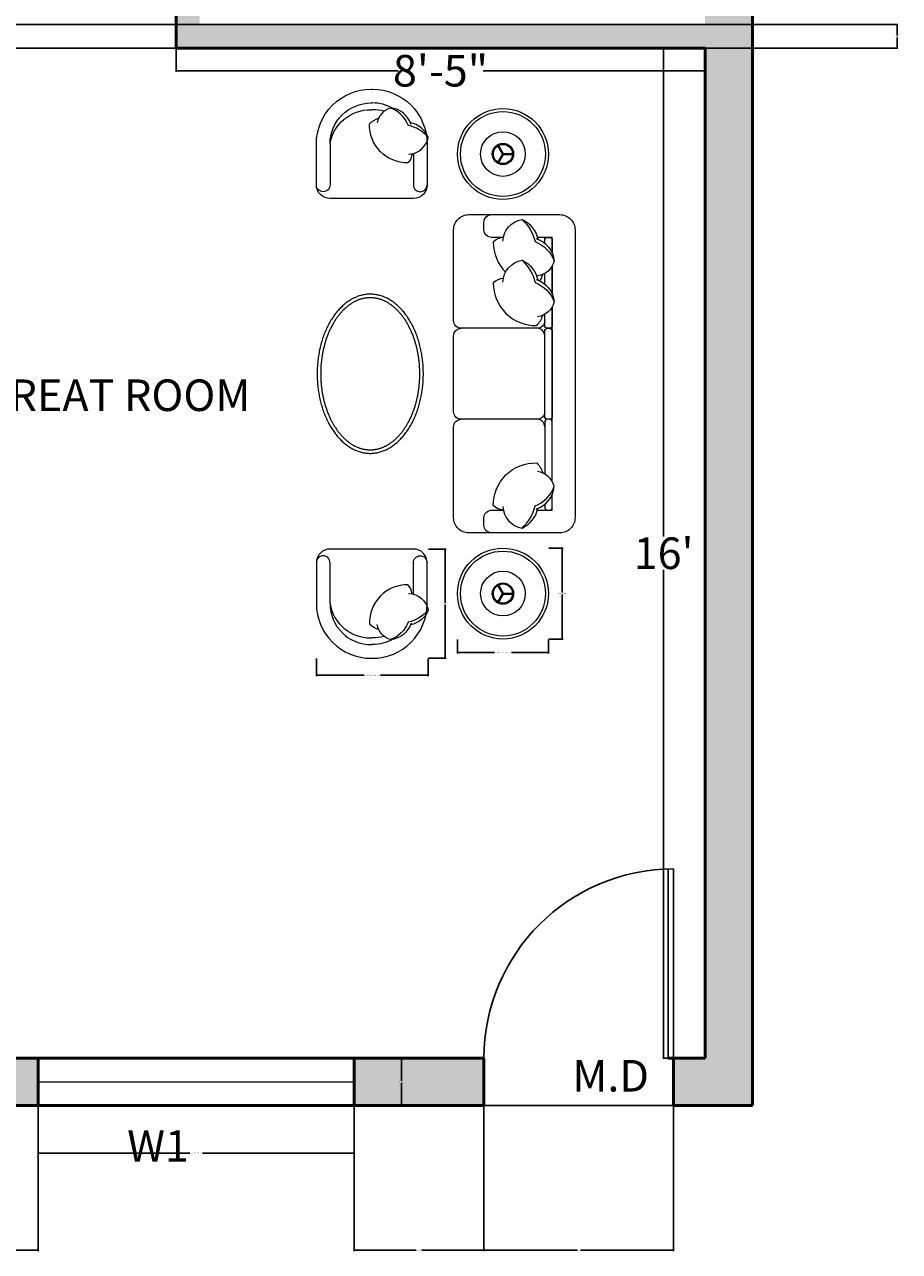
# Model space of a CAD drawing. Units: inches. Extents: x -22 to 470, y -437 to 97.
# Tile 4 of 9: x 304 to 470, y -425 to -192. Entities that reach past the tile are written whole.
import ezdxf

# ---------------------------------------------------------------- set-up
doc = ezdxf.new("R2010")
doc.units = ezdxf.units.IN
doc.header["$MEASUREMENT"] = 0
for name, color, linetype, lineweight in [('A-ANNO-DIMS', 2, 'Continuous', 18), ('A-ANNO-TEXT', 7, 'Continuous', 18), ('A-AREA-IDEN', 7, 'Continuous', 25), ('A-DOOR', 4, 'Continuous', 25), ('A-FURN', 8, 'Continuous', 18), ('A-GLAZ', 4, 'Continuous', 18), ('A-WALL', 7, 'Continuous', 50), ('A-WALL-PATT', 8, 'Continuous', 13)]:
    doc.layers.add(name, color=color, linetype=linetype, lineweight=lineweight)
doc.styles.get("Standard").update_dxf_attribs({"font": 'arial.ttf'})
doc.dimstyles.get("Standard").update_dxf_attribs({"dimtxt": 0.18, "dimasz": 0.18, "dimexe": 0.18, "dimexo": 0.0625, "dimgap": 0.09, "dimtad": 0, "dimtih": 1, "dimtoh": 1, "dimdec": 0, "dimzin": 0, "dimdsep": 46, "dimlunit": 3, "dimtxsty": 'Standard', "dimcen": 0.09, "dimadec": 0, "dimazin": 0, "dimtfac": 1, "dimtdec": 0, "dimtofl": 0, "dimtmove": 0, "dimatfit": 3, "dimfxl": 1, "dimtolj": 1, "dimtzin": 0, "dimarcsym": 0})

# ---------------------------------------------------------------- blocks, each defined once
blk = doc.blocks.new('*D21')
at = {"layer": 'A-ANNO-DIMS', "color": 0, "lineweight": -2, "transparency": 16777216}
for p, q in [((425.54, -196.94), (425.54, -289.6)), ((425.61, -196.76), (425.72, -196.76)), ((425.54, -388.58), (425.54, -295.91)), ((429.86, -388.76), (425.36, -388.76))]:
    blk.add_line(p, q, dxfattribs=at)
at = {"layer": 'A-ANNO-DIMS', "color": 0, "transparency": 16777216}
for points in [[(425.51, -196.94), (425.57, -196.94), (425.54, -196.76)], [(425.51, -388.58), (425.57, -388.58), (425.54, -388.76)]]:
    blk.add_solid(points, dxfattribs=at)
at = {"layer": 'Defpoints', "color": 0, "transparency": 16777216}
for p in [(425.54, -196.76), (425.54, -388.76), (429.92, -388.76)]:
    blk.add_point(p, dxfattribs=at)
at = {"layer": 'A-ANNO-DIMS', "color": 0, "transparency": 16777216, "insert": (425.54, -292.76), "char_height": 6, "attachment_point": 5}
blk.add_mtext("\\A1;16'", dxfattribs=at)
blk = doc.blocks.new('*D22')
at = {"layer": 'A-ANNO-DIMS', "color": 0, "lineweight": -2, "transparency": 16777216}
for p, q in [((332.92, -196.82), (332.92, -201.22)), ((433.42, -196.82), (433.42, -201.22)), ((333.1, -201.04), (375.1, -201.04)), ((433.24, -201.04), (391.24, -201.04))]:
    blk.add_line(p, q, dxfattribs=at)
at = {"layer": 'A-ANNO-DIMS', "color": 0, "transparency": 16777216}
for points in [[(333.1, -201.01), (333.1, -201.07), (332.92, -201.04)], [(433.24, -201.01), (433.24, -201.07), (433.42, -201.04)]]:
    blk.add_solid(points, dxfattribs=at)
at = {"layer": 'Defpoints', "color": 0, "transparency": 16777216}
for p in [(332.92, -196.76), (433.42, -196.76), (433.42, -201.04)]:
    blk.add_point(p, dxfattribs=at)
at = {"layer": 'A-ANNO-DIMS', "color": 0, "transparency": 16777216, "insert": (383.17, -201.04), "char_height": 6, "attachment_point": 5}
blk.add_mtext('\\A1;8\'-5"', dxfattribs=at)
blk = doc.blocks.new('ARMCHAIR')
at = {"ltscale": 0.03}
blk.add_lwpolyline([(10.52, 20.78), (2.6, 20.78, 0.414214), (0, 18.18), (0, 10.39, 0.414214), (10.39, 0), (10.52, 0), (10.65, 0, 0.414214), (21.04, 10.39), (21.04, 18.18, 0.414214), (18.44, 20.78), (10.52, 20.78)], format="xyb", dxfattribs=at)
for points in [[(2.6, 10.39), (2.6, 18.18, 0.414214), (1.3, 19.48), (1.3, 19.48, 0.414214), (0, 18.18)], [(18.44, 12.21), (18.44, 18.18, -0.414214), (19.74, 19.48), (19.74, 19.48, -0.414214), (21.04, 18.18)], [(18.19, 12.27, 0.165541), (17.38, 13.99, 0.425989), (10.09, 6.55, 0.121523), (11.82, 5.52, -7.115464)], [(17.53, 12.35, -0.356772), (21.25, 9.08, -0.249542), (17.88, 6.38, 9.61688)], [(2.6, 10.39, 0.372719), (10.39, 3.9), (10.52, 3.9)], [(2.6, 10.39, 0.414214), (10.39, 2.6), (10.52, 2.6)], [(21.25, 9.08, -0.14773), (17.46, 6.85, -0.213343), (14.11, 3.57, -0.178662)], [(17.98, 6.67, -0.306663), (14.11, 3.57, -0.30633), (11.58, 6.4, 0.872847)], [(12.86, 4.18, -0.072384), (10.65, 3.9), (10.52, 3.9)], [(14.52, 3.63, -0.130591), (10.65, 2.6), (10.52, 2.6)]]:
    blk.add_lwpolyline(points, format="xyb")
blk = doc.blocks.new('ROUND-SIDE-TABLE')
at = {"ltscale": 0.03}
for p, q in [((8.56, 8.6), (7.55, 10.36)), ((8.72, 8.69), (7.71, 10.45)), ((8.56, 8.69), (7.55, 6.93)), ((8.72, 8.6), (7.71, 6.84)), ((8.64, 8.73), (10.67, 8.73)), ((8.64, 8.55), (10.67, 8.55))]:
    blk.add_line(p, q, dxfattribs=at)
for radius in [8.64, 4.25, 2.03, 1.82]:
    blk.add_circle((8.64, 8.64), radius, dxfattribs=at)
blk.add_circle((8.64, 8.64), 8.07)
blk = doc.blocks.new('WINDOW-60-SASH')
for p, q in [((0, 9), (60, 9)), ((0, 4.5), (60, 4.5)), ((60, 0), (0, 0))]:
    blk.add_line(p, q)
blk = doc.blocks.new('*D35')
at = {"layer": 'A-ANNO-DIMS', "color": 0, "lineweight": -2, "transparency": 16777216}
for p, q in [((306.75, -397.82), (306.75, -406.94)), ((366.75, -397.82), (366.75, -406.94)), ((306.93, -406.76), (335.52, -406.76)), ((366.57, -406.76), (337.98, -406.76))]:
    blk.add_line(p, q, dxfattribs=at)
at = {"layer": 'A-ANNO-DIMS', "color": 0, "transparency": 16777216}
for points in [[(306.93, -406.73), (306.93, -406.79), (306.75, -406.76)], [(366.57, -406.73), (366.57, -406.79), (366.75, -406.76)]]:
    blk.add_solid(points, dxfattribs=at)
at = {"layer": 'Defpoints', "color": 0, "transparency": 16777216}
for p in [(306.75, -397.76), (366.75, -397.76), (366.75, -406.76)]:
    blk.add_point(p, dxfattribs=at)
at = {"layer": 'A-ANNO-DIMS', "color": 0, "transparency": 16777216, "insert": (336.75, -406.76), "char_height": 0.18, "attachment_point": 5}
blk.add_mtext('\\A1;WINDOW 5\'-0" TYP.', dxfattribs=at)
blk = doc.blocks.new('*D36')
at = {"layer": 'A-ANNO-DIMS', "color": 0, "lineweight": -2, "transparency": 16777216}
for p, q in [((366.81, -388.76), (375.93, -388.76)), ((375.75, -388.94), (375.75, -393.07)), ((375.75, -397.58), (375.75, -393.44)), ((366.81, -397.76), (375.93, -397.76))]:
    blk.add_line(p, q, dxfattribs=at)
at = {"layer": 'A-ANNO-DIMS', "color": 0, "transparency": 16777216}
for points in [[(375.72, -388.94), (375.78, -388.94), (375.75, -388.76)], [(375.72, -397.58), (375.78, -397.58), (375.75, -397.76)]]:
    blk.add_solid(points, dxfattribs=at)
at = {"layer": 'Defpoints', "color": 0, "transparency": 16777216}
for p in [(366.75, -388.76), (375.75, -388.76), (366.75, -397.76)]:
    blk.add_point(p, dxfattribs=at)
at = {"layer": 'A-ANNO-DIMS', "color": 0, "transparency": 16777216, "insert": (375.75, -393.26), "char_height": 0.18, "attachment_point": 5}
blk.add_mtext('\\A1;0\'-9" TYP.', dxfattribs=at)
blk = doc.blocks.new('*D47')
at = {"layer": 'A-ANNO-DIMS', "color": 0, "lineweight": -2, "transparency": 16777216}
for p, q in [((359.58, -312.79), (359.58, -316.1)), ((380.84, -312.79), (380.84, -316.1)), ((359.76, -315.92), (368.65, -315.92)), ((380.66, -315.92), (371.77, -315.92))]:
    blk.add_line(p, q, dxfattribs=at)
at = {"layer": 'A-ANNO-DIMS', "color": 0, "transparency": 16777216}
for points in [[(359.76, -315.89), (359.76, -315.95), (359.58, -315.92)], [(380.66, -315.89), (380.66, -315.95), (380.84, -315.92)]]:
    blk.add_solid(points, dxfattribs=at)
at = {"layer": 'Defpoints', "color": 0, "transparency": 16777216}
for p in [(359.58, -312.73), (380.84, -312.73), (380.84, -315.92)]:
    blk.add_point(p, dxfattribs=at)
at = {"layer": 'A-ANNO-DIMS', "color": 0, "transparency": 16777216, "insert": (370.21, -315.92), "char_height": 0.18, "attachment_point": 5}
blk.add_mtext('\\A1;ARMCHAIR 1\'-9 1/2" TYP.', dxfattribs=at)
blk = doc.blocks.new('*D48')
at = {"layer": 'A-ANNO-DIMS', "color": 0, "lineweight": -2, "transparency": 16777216}
for p, q in [((380.9, -291.95), (384.21, -291.95)), ((384.03, -292.13), (384.03, -302.16)), ((384.03, -312.55), (384.03, -302.52)), ((380.9, -312.73), (384.21, -312.73))]:
    blk.add_line(p, q, dxfattribs=at)
at = {"layer": 'A-ANNO-DIMS', "color": 0, "transparency": 16777216}
for points in [[(384, -292.13), (384.06, -292.13), (384.03, -291.95)], [(384, -312.55), (384.06, -312.55), (384.03, -312.73)]]:
    blk.add_solid(points, dxfattribs=at)
at = {"layer": 'Defpoints', "color": 0, "transparency": 16777216}
for p in [(380.84, -291.95), (384.03, -291.95), (380.84, -312.73)]:
    blk.add_point(p, dxfattribs=at)
at = {"layer": 'A-ANNO-DIMS', "color": 0, "transparency": 16777216, "insert": (384.03, -302.34), "char_height": 0.18, "attachment_point": 5}
blk.add_mtext('\\A1;1\'-9" TYP.', dxfattribs=at)
blk = doc.blocks.new('*D49')
at = {"layer": 'A-ANNO-DIMS', "color": 0, "lineweight": -2, "transparency": 16777216}
for p, q in [((386.38, -309.12), (386.38, -311.83)), ((403.67, -309.12), (403.67, -311.83)), ((386.56, -311.65), (393.42, -311.65)), ((403.49, -311.65), (396.63, -311.65))]:
    blk.add_line(p, q, dxfattribs=at)
at = {"layer": 'A-ANNO-DIMS', "color": 0, "transparency": 16777216}
for points in [[(386.56, -311.62), (386.56, -311.68), (386.38, -311.65)], [(403.49, -311.62), (403.49, -311.68), (403.67, -311.65)]]:
    blk.add_solid(points, dxfattribs=at)
at = {"layer": 'Defpoints', "color": 0, "transparency": 16777216}
for p in [(386.38, -309.06), (403.67, -309.06), (403.67, -311.65)]:
    blk.add_point(p, dxfattribs=at)
at = {"layer": 'A-ANNO-DIMS', "color": 0, "transparency": 16777216, "insert": (395.02, -311.65), "char_height": 0.18, "attachment_point": 5}
blk.add_mtext('\\A1;SIDE TABLE 1\'-5 1/2" TYP.', dxfattribs=at)
blk = doc.blocks.new('*D50')
at = {"layer": 'A-ANNO-DIMS', "color": 0, "lineweight": -2, "transparency": 16777216}
for p, q in [((403.73, -291.77), (406.44, -291.77)), ((406.26, -291.95), (406.26, -300.23)), ((406.26, -308.88), (406.26, -300.6)), ((403.73, -309.06), (406.44, -309.06))]:
    blk.add_line(p, q, dxfattribs=at)
at = {"layer": 'A-ANNO-DIMS', "color": 0, "transparency": 16777216}
for points in [[(406.23, -291.95), (406.29, -291.95), (406.26, -291.77)], [(406.23, -308.88), (406.29, -308.88), (406.26, -309.06)]]:
    blk.add_solid(points, dxfattribs=at)
at = {"layer": 'Defpoints', "color": 0, "transparency": 16777216}
for p in [(403.67, -291.77), (406.26, -291.77), (403.67, -309.06)]:
    blk.add_point(p, dxfattribs=at)
at = {"layer": 'A-ANNO-DIMS', "color": 0, "transparency": 16777216, "insert": (406.26, -300.42), "char_height": 0.18, "attachment_point": 5}
blk.add_mtext('\\A1;1\'-5 1/2" TYP.', dxfattribs=at)
blk = doc.blocks.new('*D61')
at = {"layer": 'A-ANNO-DIMS', "color": 0, "lineweight": -2, "transparency": 16777216}
for p, q in [((391.42, -388.82), (391.42, -425.39)), ((427.42, -388.82), (427.42, -425.39)), ((391.6, -425.21), (409.09, -425.21)), ((427.24, -425.21), (409.75, -425.21))]:
    blk.add_line(p, q, dxfattribs=at)
at = {"layer": 'A-ANNO-DIMS', "color": 0, "transparency": 16777216}
for points in [[(391.6, -425.18), (391.6, -425.24), (391.42, -425.21)], [(427.24, -425.18), (427.24, -425.24), (427.42, -425.21)]]:
    blk.add_solid(points, dxfattribs=at)
at = {"layer": 'Defpoints', "color": 0, "transparency": 16777216}
for p in [(391.42, -388.76), (427.42, -388.76), (427.42, -425.21)]:
    blk.add_point(p, dxfattribs=at)
at = {"layer": 'A-ANNO-DIMS', "color": 0, "transparency": 16777216, "insert": (409.42, -425.21), "char_height": 0.18, "attachment_point": 5}
blk.add_mtext('\\A1;3\'-0"', dxfattribs=at)
blk = doc.blocks.new('*D64')
at = {"layer": 'A-ANNO-DIMS', "color": 0, "lineweight": -2, "transparency": 16777216}
for p, q in [((168.98, -192.26), (470.05, -192.26)), ((469.87, -192.44), (469.87, -194.32)), ((469.87, -196.58), (469.87, -194.69)), ((168.98, -196.76), (470.05, -196.76))]:
    blk.add_line(p, q, dxfattribs=at)
at = {"layer": 'A-ANNO-DIMS', "color": 0, "transparency": 16777216}
for points in [[(469.84, -192.44), (469.9, -192.44), (469.87, -192.26)], [(469.84, -196.58), (469.9, -196.58), (469.87, -196.76)]]:
    blk.add_solid(points, dxfattribs=at)
at = {"layer": 'Defpoints', "color": 0, "transparency": 16777216}
for p in [(168.92, -192.26), (168.92, -196.76), (469.87, -196.76)]:
    blk.add_point(p, dxfattribs=at)
at = {"layer": 'A-ANNO-DIMS', "color": 0, "transparency": 16777216, "insert": (469.87, -194.51), "char_height": 0.18, "attachment_point": 5}
blk.add_mtext('\\A1;0\'-4 1/2"', dxfattribs=at)
blk = doc.blocks.new('*D75')
at = {"layer": 'A-ANNO-DIMS', "color": 0, "lineweight": -2, "transparency": 16777216}
for p, q in [((278.92, -397.82), (278.92, -425.39)), ((306.75, -397.82), (306.75, -425.39)), ((279.1, -425.21), (292.51, -425.21)), ((306.57, -425.21), (293.17, -425.21))]:
    blk.add_line(p, q, dxfattribs=at)
at = {"layer": 'A-ANNO-DIMS', "color": 0, "transparency": 16777216}
for points in [[(279.1, -425.18), (279.1, -425.24), (278.92, -425.21)], [(306.57, -425.18), (306.57, -425.24), (306.75, -425.21)]]:
    blk.add_solid(points, dxfattribs=at)
at = {"layer": 'Defpoints', "color": 0, "transparency": 16777216}
for p in [(278.92, -397.76), (306.75, -397.76), (306.75, -425.21)]:
    blk.add_point(p, dxfattribs=at)
at = {"layer": 'A-ANNO-DIMS', "color": 0, "transparency": 16777216, "insert": (292.84, -425.21), "char_height": 0.18, "attachment_point": 5}
blk.add_mtext('\\A1;2\'-4"', dxfattribs=at)
blk = doc.blocks.new('*D76')
at = {"layer": 'A-ANNO-DIMS', "color": 0, "lineweight": -2, "transparency": 16777216}
for p, q in [((366.75, -397.82), (366.75, -425.39)), ((391.42, -397.82), (391.42, -425.39)), ((366.93, -425.21), (378.55, -425.21)), ((391.24, -425.21), (379.63, -425.21))]:
    blk.add_line(p, q, dxfattribs=at)
at = {"layer": 'A-ANNO-DIMS', "color": 0, "transparency": 16777216}
for points in [[(366.93, -425.18), (366.93, -425.24), (366.75, -425.21)], [(391.24, -425.18), (391.24, -425.24), (391.42, -425.21)]]:
    blk.add_solid(points, dxfattribs=at)
at = {"layer": 'Defpoints', "color": 0, "transparency": 16777216}
for p in [(366.75, -397.76), (391.42, -397.76), (391.42, -425.21)]:
    blk.add_point(p, dxfattribs=at)
at = {"layer": 'A-ANNO-DIMS', "color": 0, "transparency": 16777216, "insert": (379.09, -425.21), "char_height": 0.18, "attachment_point": 5}
blk.add_mtext('\\A1;2\'-0 1/2"', dxfattribs=at)

msp = doc.modelspace()

# ---------------------------------------------------------------- hatches: boundary and pattern name
at = {"layer": 'A-WALL-PATT'}
h = msp.add_hatch(color=256, dxfattribs=at)
h.dxf.hatch_style = 1
h.paths.add_polyline_path([(130.42, 13.24), (26.92, 13.24), (26.92, -43.76), (35.92, -43.76), (35.92, 4.24), (83.92, 4.24), (83.92, 1.24), (88.42, 1.24), (88.42, 4.24), (130.42, 4.24)])
h.paths.add_polyline_path([(266.92, 13.24), (190.42, 13.24), (190.42, 4.24), (232.42, 4.24), (232.42, -115.76), (229.42, -115.76), (229.42, -120.26), (239.92, -120.26), (239.92, -115.76), (236.92, -115.76), (236.92, 4.24), (266.92, 4.24)])
h.paths.add_polyline_path([(442.42, 13.24), (326.92, 13.24), (326.92, 4.24), (356.92, 4.24), (356.92, 1.24), (361.42, 1.24), (361.42, 4.24), (433.42, 4.24), (433.42, -49.38), (442.42, -49.38)])
h.paths.add_polyline_path([(442.42, -73.38), (433.42, -73.38), (433.42, -115.76), (361.42, -115.76), (361.42, -22.76), (356.92, -22.76), (356.92, -115.76), (263.92, -115.76), (263.92, -120.26), (332.92, -120.26), (332.92, -123.26), (337.42, -123.26), (337.42, -120.26), (433.42, -120.26), (433.42, -148.49), (442.42, -148.49)])
h.paths.add_polyline_path([(205.42, -115.76), (88.42, -115.76), (88.42, -22.76), (83.92, -22.76), (83.92, -115.76), (35.92, -115.76), (35.92, -67.76), (26.92, -67.76), (26.92, -126.26), (35.92, -126.26), (35.92, -120.26), (205.42, -120.26)])
h.paths.add_polyline_path([(35.92, -196.76), (168.92, -196.76), (168.92, -192.26), (35.92, -192.26), (35.92, -186.26), (26.92, -186.26), (26.92, -224.25), (35.92, -224.25)])
h.paths.add_polyline_path([(35.92, -284.25), (26.92, -284.25), (26.92, -397.76), (53.92, -397.76), (53.92, -388.76), (35.92, -388.76)])
h.paths.add_polyline_path([(142.42, -388.76), (136.42, -388.76), (136.42, -316.76), (181.42, -316.76), (181.42, -312.26), (136.42, -312.26), (136.42, -303.75), (131.92, -303.75), (131.92, -388.76), (113.92, -388.76), (113.92, -397.76), (142.42, -397.76)])
h.paths.add_polyline_path([(218.92, -388.76), (212.92, -388.76), (212.92, -312.26), (205.42, -312.26), (205.42, -316.76), (208.42, -316.76), (208.42, -388.76), (202.42, -388.76), (202.42, -397.76), (218.92, -397.76)])
h.paths.add_polyline_path([(306.75, -388.76), (289.42, -388.76), (289.42, -316.76), (284.92, -316.76), (284.92, -388.76), (278.92, -388.76), (278.92, -397.76), (306.75, -397.76)])
h.paths.add_polyline_path([(391.42, -388.76), (366.75, -388.76), (366.75, -397.76), (391.42, -397.76)], flags=17)
h.paths.add_polyline_path([(442.42, -172.49), (433.42, -172.49), (433.42, -192.26), (337.42, -192.26), (337.42, -147.26), (332.92, -147.26), (332.92, -196.76), (433.42, -196.76), (433.42, -388.76), (427.42, -388.76), (427.42, -397.76), (442.42, -397.76)])

# ---------------------------------------------------------------- linework, layer by layer
at = {"layer": 'A-DOOR'}
for p, q in [((426.42, -388.76), (426.42, -352.76)), ((427.42, -388.76), (427.42, -352.76)), ((391.42, -397.76), (427.42, -397.76))]:
    msp.add_line(p, q, dxfattribs=at)
msp.add_arc((427.42, -388.76), 36, 90, 180, dxfattribs=at)
at = {"layer": 'A-FURN', "ltscale": 0.03}
msp.add_lwpolyline([(388.54, -288.89, -0.414214), (385.66, -286.01), (385.66, -268.73, -0.414214), (387.1, -267.29, -0.414214), (385.66, -265.85), (385.66, -251.44, -0.414214), (387.1, -250, -0.414214), (385.66, -248.56), (385.66, -231.27, -0.414214), (388.54, -228.39), (405.83, -228.39, -0.414214), (408.71, -231.27), (408.71, -286.01, -0.414214), (405.83, -288.89)], format="xyb", close=True, dxfattribs=at)
at = {"layer": 'A-FURN'}
for points in [[(395.1, -232.71), (392.86, -232.71, -0.414214), (391.42, -231.27), (391.42, -229.83, -0.414214), (392.86, -228.39)], [(395.01, -233.44, -0.356772), (398.64, -229.31, -0.249542), (401.63, -233.05, 9.61688)], [(398.64, -229.31, -0.14773), (401.12, -233.52, -0.213343), (404.75, -237.23, -0.178662)], [(395.1, -232.71, 0.165541), (393.19, -233.6, 0.200231), (395.51, -239.32, 0.121523)], [(401.31, -232.94, -0.306663), (404.75, -237.23, -0.30633), (401.61, -240.04, 0.872847)], [(404.39, -235.74), (404.39, -232.71), (401.56, -232.71, -0.414214)], [(402.95, -233.81), (402.95, -233.29, -0.414214), (403.52, -232.71), (403.81, -232.71, -0.414214), (404.39, -233.29)], [(404.39, -233.29), (404.39, -235.74, -0.414214)], [(395.01, -241.2, -0.356772), (398.64, -237.07, -0.249542), (401.63, -240.81, 9.61688)], [(398.64, -237.07, -0.14773), (401.12, -241.28, -0.213343), (404.75, -244.99, -0.178662)], [(402.02, -240.98, 0.071865), (402.58, -239.77, -7.115464)], [(402.95, -241.57), (402.95, -239.59, -0.414214)], [(404.39, -238.14), (404.39, -243.5, -0.414214)], [(395.1, -240.47, 0.165541), (393.19, -241.36, 0.425989), (401.45, -249.45, 0.121523), (402.58, -247.53, -7.115464)], [(401.31, -240.7, -0.306663), (404.75, -244.99, -0.30633), (401.61, -247.8, 0.872847)], [(404.39, -245.9), (404.39, -249.42, -0.414214), (403.81, -250), (403.52, -250, -0.414214), (402.95, -249.42), (402.95, -247.35, -0.414214)], [(402.95, -248.56, -0.414214), (401.51, -250), (387.1, -250, -0.414214)], [(402.95, -251.44, 0.414214), (401.51, -250)], [(402.95, -265.85, -0.414214), (401.51, -267.29)], [(402.95, -268.73, 0.414214), (401.51, -267.29), (387.1, -267.29, 0.414214)], [(404.39, -279.14), (404.39, -267.86, 0.414214), (403.81, -267.29), (403.52, -267.29, 0.414214), (402.95, -267.86), (402.95, -277.69, 0.414214)], [(395.1, -284.57, -0.165541), (393.19, -283.68, -0.425989), (401.45, -275.59, -0.121523), (402.58, -277.51, 7.115464)], [(401.31, -284.35, 0.306663), (404.75, -280.05, 0.30633), (401.61, -277.24, -0.872847)], [(398.64, -287.98, 0.14773), (401.12, -283.77, 0.213343), (404.75, -280.05, 0.178662)], [(404.39, -284), (404.39, -281.54, 0.414214)], [(395.01, -283.85, 0.356772), (398.64, -287.98, 0.249542), (401.63, -284.24, -9.61688)], [(402.95, -283.47), (402.95, -284, 0.414214), (403.52, -284.57), (403.81, -284.57, 0.414214), (404.39, -284)], [(392.86, -288.89, -0.414214), (391.42, -287.45), (391.42, -286.01, -0.414214), (392.86, -284.57), (395.1, -284.57)]]:
    msp.add_lwpolyline(points, format="xyb", dxfattribs=at)
for points in [[(404.39, -243.5), (404.39, -238.14)], [(404.39, -279.14), (404.39, -245.9)], [(401.56, -284.57), (404.39, -284.57), (404.39, -281.54)]]:
    msp.add_lwpolyline(points, dxfattribs=at)
msp.add_lwpolyline([(404.39, -250.58), (404.39, -266.71, -0.414214), (403.81, -267.29), (403.52, -267.29, -0.414214), (402.95, -266.71), (402.95, -250.58, -0.414214), (403.52, -250), (403.81, -250, -0.414214)], format="xyb", close=True, dxfattribs=at)
at = {"layer": 'A-FURN', "ltscale": 0.03}
msp.add_polyline3d([(369.82, -273.77, 0), (370.01, -273.77, 0), (370.2, -273.76, 0), (370.39, -273.74, 0), (370.58, -273.72, 0), (370.77, -273.7, 0), (370.96, -273.67, 0), (371.15, -273.64, 0), (371.34, -273.59, 0), (371.53, -273.55, 0), (371.71, -273.5, 0), (371.9, -273.44, 0), (372.09, -273.38, 0), (372.27, -273.31, 0), (372.46, -273.24, 0), (372.64, -273.16, 0), (372.82, -273.08, 0), (373.01, -272.99, 0), (373.19, -272.9, 0), (373.36, -272.8, 0), (373.54, -272.7, 0), (373.72, -272.59, 0), (373.89, -272.48, 0), (374.07, -272.36, 0), (374.24, -272.23, 0), (374.41, -272.11, 0), (374.58, -271.97, 0), (374.75, -271.84, 0), (374.91, -271.69, 0), (375.08, -271.55, 0), (375.24, -271.39, 0), (375.4, -271.24, 0), (375.56, -271.08, 0), (375.71, -270.91, 0), (375.87, -270.74, 0), (376.02, -270.57, 0), (376.17, -270.39, 0), (376.31, -270.21, 0), (376.46, -270.02, 0), (376.6, -269.83, 0), (376.74, -269.64, 0), (376.88, -269.44, 0), (377.01, -269.24, 0), (377.15, -269.03, 0), (377.28, -268.82, 0), (377.4, -268.61, 0), (377.53, -268.39, 0), (377.65, -268.17, 0), (377.77, -267.94, 0), (377.88, -267.72, 0), (378, -267.49, 0), (378.11, -267.25, 0), (378.21, -267.02, 0), (378.32, -266.78, 0), (378.42, -266.53, 0), (378.52, -266.29, 0), (378.61, -266.04, 0), (378.7, -265.79, 0), (378.79, -265.53, 0), (378.88, -265.28, 0), (378.96, -265.02, 0), (379.04, -264.76, 0), (379.11, -264.5, 0), (379.19, -264.23, 0), (379.26, -263.97, 0), (379.32, -263.7, 0), (379.38, -263.43, 0), (379.44, -263.15, 0), (379.5, -262.88, 0), (379.55, -262.6, 0), (379.6, -262.33, 0), (379.64, -262.05, 0), (379.68, -261.77, 0), (379.72, -261.49, 0), (379.75, -261.21, 0), (379.78, -260.92, 0), (379.81, -260.64, 0), (379.84, -260.36, 0), (379.85, -260.07, 0), (379.87, -259.79, 0), (379.88, -259.5, 0), (379.89, -259.22, 0), (379.9, -258.93, 0), (379.9, -258.64, 0), (379.9, -258.36, 0), (379.89, -258.07, 0), (379.88, -257.78, 0), (379.87, -257.5, 0), (379.85, -257.21, 0), (379.84, -256.93, 0), (379.81, -256.65, 0), (379.78, -256.36, 0), (379.75, -256.08, 0), (379.72, -255.8, 0), (379.68, -255.52, 0), (379.64, -255.24, 0), (379.6, -254.96, 0), (379.55, -254.68, 0), (379.5, -254.41, 0), (379.44, -254.13, 0), (379.38, -253.86, 0), (379.32, -253.59, 0), (379.26, -253.32, 0), (379.19, -253.05, 0), (379.11, -252.79, 0), (379.04, -252.53, 0), (378.96, -252.27, 0), (378.88, -252.01, 0), (378.79, -251.75, 0), (378.7, -251.5, 0), (378.61, -251.25, 0), (378.52, -251, 0), (378.42, -250.75, 0), (378.32, -250.51, 0), (378.21, -250.27, 0), (378.11, -250.03, 0), (378, -249.8, 0), (377.88, -249.57, 0), (377.77, -249.34, 0), (377.65, -249.12, 0), (377.53, -248.9, 0), (377.4, -248.68, 0), (377.28, -248.47, 0), (377.15, -248.26, 0), (377.01, -248.05, 0), (376.88, -247.85, 0), (376.74, -247.65, 0), (376.6, -247.45, 0), (376.46, -247.26, 0), (376.31, -247.08, 0), (376.17, -246.89, 0), (376.02, -246.72, 0), (375.87, -246.54, 0), (375.71, -246.37, 0), (375.56, -246.21, 0), (375.4, -246.05, 0), (375.24, -245.89, 0), (375.08, -245.74, 0), (374.91, -245.59, 0), (374.75, -245.45, 0), (374.58, -245.31, 0), (374.41, -245.18, 0), (374.24, -245.05, 0), (374.07, -244.93, 0), (373.89, -244.81, 0), (373.72, -244.7, 0), (373.54, -244.59, 0), (373.36, -244.49, 0), (373.19, -244.39, 0), (373.01, -244.29, 0), (372.82, -244.21, 0), (372.64, -244.12, 0), (372.46, -244.05, 0), (372.27, -243.97, 0), (372.09, -243.91, 0), (371.9, -243.84, 0), (371.71, -243.79, 0), (371.53, -243.74, 0), (371.34, -243.69, 0), (371.15, -243.65, 0), (370.96, -243.62, 0), (370.77, -243.59, 0), (370.58, -243.56, 0), (370.39, -243.54, 0), (370.2, -243.53, 0), (370.01, -243.52, 0), (369.82, -243.52, 0), (369.63, -243.52, 0), (369.44, -243.53, 0), (369.24, -243.54, 0), (369.05, -243.56, 0), (368.86, -243.59, 0), (368.67, -243.62, 0), (368.48, -243.65, 0), (368.3, -243.69, 0), (368.11, -243.74, 0), (367.92, -243.79, 0), (367.73, -243.84, 0), (367.55, -243.91, 0), (367.36, -243.97, 0), (367.18, -244.05, 0), (366.99, -244.12, 0), (366.81, -244.21, 0), (366.63, -244.29, 0), (366.45, -244.39, 0), (366.27, -244.49, 0), (366.09, -244.59, 0), (365.91, -244.7, 0), (365.74, -244.81, 0), (365.56, -244.93, 0), (365.39, -245.05, 0), (365.22, -245.18, 0), (365.05, -245.31, 0), (364.89, -245.45, 0), (364.72, -245.59, 0), (364.56, -245.74, 0), (364.39, -245.89, 0), (364.23, -246.05, 0), (364.08, -246.21, 0), (363.92, -246.37, 0), (363.77, -246.54, 0), (363.62, -246.72, 0), (363.47, -246.89, 0), (363.32, -247.08, 0), (363.17, -247.26, 0), (363.03, -247.45, 0), (362.89, -247.65, 0), (362.75, -247.85, 0), (362.62, -248.05, 0), (362.49, -248.26, 0), (362.36, -248.47, 0), (362.23, -248.68, 0), (362.11, -248.9, 0), (361.98, -249.12, 0), (361.87, -249.34, 0), (361.75, -249.57, 0), (361.64, -249.8, 0), (361.53, -250.03, 0), (361.42, -250.27, 0), (361.32, -250.51, 0), (361.21, -250.75, 0), (361.12, -251, 0), (361.02, -251.25, 0), (360.93, -251.5, 0), (360.84, -251.75, 0), (360.76, -252.01, 0), (360.67, -252.27, 0), (360.59, -252.53, 0), (360.52, -252.79, 0), (360.45, -253.05, 0), (360.38, -253.32, 0), (360.31, -253.59, 0), (360.25, -253.86, 0), (360.19, -254.13, 0), (360.14, -254.41, 0), (360.09, -254.68, 0), (360.04, -254.96, 0), (359.99, -255.24, 0), (359.95, -255.52, 0), (359.91, -255.8, 0), (359.88, -256.08, 0), (359.85, -256.36, 0), (359.82, -256.65, 0), (359.8, -256.93, 0), (359.78, -257.21, 0), (359.76, -257.5, 0), (359.75, -257.78, 0), (359.74, -258.07, 0), (359.74, -258.36, 0), (359.73, -258.64, 0), (359.74, -258.93, 0), (359.74, -259.22, 0), (359.75, -259.5, 0), (359.76, -259.79, 0), (359.78, -260.07, 0), (359.8, -260.36, 0), (359.82, -260.64, 0), (359.85, -260.92, 0), (359.88, -261.21, 0), (359.91, -261.49, 0), (359.95, -261.77, 0), (359.99, -262.05, 0), (360.04, -262.33, 0), (360.09, -262.6, 0), (360.14, -262.88, 0), (360.19, -263.15, 0), (360.25, -263.43, 0), (360.31, -263.7, 0), (360.38, -263.97, 0), (360.45, -264.23, 0), (360.52, -264.5, 0), (360.59, -264.76, 0), (360.67, -265.02, 0), (360.76, -265.28, 0), (360.84, -265.53, 0), (360.93, -265.79, 0), (361.02, -266.04, 0), (361.12, -266.29, 0), (361.21, -266.53, 0), (361.32, -266.78, 0), (361.42, -267.02, 0), (361.53, -267.25, 0), (361.64, -267.49, 0), (361.75, -267.72, 0), (361.87, -267.94, 0), (361.98, -268.17, 0), (362.11, -268.39, 0), (362.23, -268.61, 0), (362.36, -268.82, 0), (362.49, -269.03, 0), (362.62, -269.24, 0), (362.75, -269.44, 0), (362.89, -269.64, 0), (363.03, -269.83, 0), (363.17, -270.02, 0), (363.32, -270.21, 0), (363.47, -270.39, 0), (363.62, -270.57, 0), (363.77, -270.74, 0), (363.92, -270.91, 0), (364.08, -271.08, 0), (364.23, -271.24, 0), (364.39, -271.39, 0), (364.56, -271.55, 0), (364.72, -271.69, 0), (364.89, -271.84, 0), (365.05, -271.97, 0), (365.22, -272.11, 0), (365.39, -272.23, 0), (365.56, -272.36, 0), (365.74, -272.48, 0), (365.91, -272.59, 0), (366.09, -272.7, 0), (366.27, -272.8, 0), (366.45, -272.9, 0), (366.63, -272.99, 0), (366.81, -273.08, 0), (366.99, -273.16, 0), (367.18, -273.24, 0), (367.36, -273.31, 0), (367.55, -273.38, 0), (367.73, -273.44, 0), (367.92, -273.5, 0), (368.11, -273.55, 0), (368.3, -273.59, 0), (368.48, -273.64, 0), (368.67, -273.67, 0), (368.86, -273.7, 0), (369.05, -273.72, 0), (369.24, -273.74, 0), (369.44, -273.76, 0), (369.63, -273.77, 0), (369.82, -273.77, 0)], dxfattribs=at)
at = {"layer": 'A-FURN'}
msp.add_polyline3d([(369.82, -273.1, 0), (369.92, -273.09, 0), (370.02, -273.09, 0), (370.13, -273.09, 0), (370.23, -273.08, 0), (370.34, -273.07, 0), (370.44, -273.06, 0), (370.55, -273.05, 0), (370.65, -273.04, 0), (370.76, -273.02, 0), (370.87, -273, 0), (370.97, -272.98, 0), (371.08, -272.96, 0), (371.19, -272.94, 0), (371.3, -272.91, 0), (371.41, -272.89, 0), (371.52, -272.86, 0), (371.62, -272.82, 0), (371.73, -272.79, 0), (371.84, -272.75, 0), (371.95, -272.71, 0), (372.06, -272.67, 0), (372.17, -272.63, 0), (372.28, -272.58, 0), (372.39, -272.54, 0), (372.5, -272.49, 0), (372.61, -272.43, 0), (372.72, -272.38, 0), (372.84, -272.32, 0), (372.95, -272.26, 0), (373.06, -272.2, 0), (373.17, -272.14, 0), (373.28, -272.07, 0), (373.39, -272, 0), (373.5, -271.93, 0), (373.6, -271.86, 0), (373.71, -271.79, 0), (373.82, -271.71, 0), (373.93, -271.63, 0), (374.04, -271.54, 0), (374.15, -271.46, 0), (374.25, -271.37, 0), (374.36, -271.28, 0), (374.47, -271.19, 0), (374.57, -271.1, 0), (374.68, -271, 0), (374.78, -270.9, 0), (374.88, -270.8, 0), (374.99, -270.7, 0), (375.09, -270.59, 0), (375.19, -270.48, 0), (375.29, -270.37, 0), (375.39, -270.26, 0), (375.49, -270.14, 0), (375.59, -270.02, 0), (375.69, -269.9, 0), (375.79, -269.78, 0), (375.88, -269.66, 0), (375.98, -269.53, 0), (376.07, -269.4, 0), (376.16, -269.27, 0), (376.26, -269.14, 0), (376.35, -269.01, 0), (376.44, -268.87, 0), (376.53, -268.74, 0), (376.61, -268.6, 0), (376.7, -268.46, 0), (376.79, -268.31, 0), (376.87, -268.17, 0), (376.95, -268.02, 0), (377.03, -267.88, 0), (377.12, -267.73, 0), (377.19, -267.58, 0), (377.27, -267.43, 0), (377.35, -267.27, 0), (377.42, -267.12, 0), (377.5, -266.96, 0), (377.57, -266.8, 0), (377.64, -266.64, 0), (377.71, -266.48, 0), (377.78, -266.32, 0), (377.84, -266.16, 0), (377.91, -266, 0), (377.97, -265.83, 0), (378.03, -265.67, 0), (378.09, -265.5, 0), (378.15, -265.33, 0), (378.21, -265.17, 0), (378.26, -265, 0), (378.32, -264.83, 0), (378.37, -264.66, 0), (378.42, -264.49, 0), (378.47, -264.32, 0), (378.51, -264.15, 0), (378.56, -263.98, 0), (378.6, -263.81, 0), (378.64, -263.64, 0), (378.69, -263.47, 0), (378.72, -263.3, 0), (378.76, -263.13, 0), (378.8, -262.96, 0), (378.83, -262.79, 0), (378.87, -262.61, 0), (378.9, -262.44, 0), (378.93, -262.27, 0), (378.96, -262.09, 0), (378.98, -261.92, 0), (379.01, -261.75, 0), (379.03, -261.57, 0), (379.06, -261.4, 0), (379.08, -261.23, 0), (379.1, -261.05, 0), (379.12, -260.88, 0), (379.13, -260.7, 0), (379.15, -260.53, 0), (379.16, -260.35, 0), (379.18, -260.18, 0), (379.19, -260, 0), (379.2, -259.83, 0), (379.21, -259.65, 0), (379.21, -259.48, 0), (379.22, -259.3, 0), (379.22, -259.13, 0), (379.23, -258.95, 0), (379.23, -258.77, 0), (379.23, -258.6, 0), (379.23, -258.42, 0), (379.22, -258.25, 0), (379.22, -258.07, 0), (379.22, -257.9, 0), (379.21, -257.72, 0), (379.2, -257.55, 0), (379.19, -257.37, 0), (379.18, -257.2, 0), (379.17, -257.02, 0), (379.16, -256.85, 0), (379.14, -256.67, 0), (379.12, -256.5, 0), (379.11, -256.32, 0), (379.09, -256.15, 0), (379.07, -255.97, 0), (379.05, -255.8, 0), (379.02, -255.63, 0), (379, -255.45, 0), (378.97, -255.28, 0), (378.94, -255.1, 0), (378.91, -254.93, 0), (378.88, -254.76, 0), (378.85, -254.59, 0), (378.82, -254.41, 0), (378.78, -254.24, 0), (378.74, -254.07, 0), (378.71, -253.9, 0), (378.67, -253.73, 0), (378.62, -253.56, 0), (378.58, -253.39, 0), (378.54, -253.22, 0), (378.49, -253.05, 0), (378.44, -252.88, 0), (378.39, -252.71, 0), (378.34, -252.54, 0), (378.29, -252.37, 0), (378.24, -252.2, 0), (378.18, -252.04, 0), (378.12, -251.87, 0), (378.06, -251.7, 0), (378, -251.54, 0), (377.94, -251.37, 0), (377.88, -251.21, 0), (377.81, -251.04, 0), (377.74, -250.88, 0), (377.68, -250.72, 0), (377.61, -250.56, 0), (377.53, -250.4, 0), (377.46, -250.25, 0), (377.39, -250.09, 0), (377.31, -249.94, 0), (377.23, -249.78, 0), (377.16, -249.63, 0), (377.08, -249.48, 0), (376.99, -249.34, 0), (376.91, -249.19, 0), (376.83, -249.04, 0), (376.74, -248.9, 0), (376.66, -248.76, 0), (376.57, -248.62, 0), (376.48, -248.48, 0), (376.39, -248.34, 0), (376.3, -248.21, 0), (376.21, -248.08, 0), (376.12, -247.95, 0), (376.02, -247.82, 0), (375.93, -247.69, 0), (375.83, -247.57, 0), (375.74, -247.44, 0), (375.64, -247.32, 0), (375.54, -247.2, 0), (375.44, -247.09, 0), (375.34, -246.97, 0), (375.24, -246.86, 0), (375.14, -246.75, 0), (375.04, -246.64, 0), (374.94, -246.54, 0), (374.83, -246.44, 0), (374.73, -246.33, 0), (374.62, -246.24, 0), (374.52, -246.14, 0), (374.41, -246.05, 0), (374.31, -245.96, 0), (374.2, -245.87, 0), (374.09, -245.78, 0), (373.98, -245.7, 0), (373.88, -245.62, 0), (373.77, -245.54, 0), (373.66, -245.46, 0), (373.55, -245.39, 0), (373.44, -245.32, 0), (373.33, -245.25, 0), (373.22, -245.18, 0), (373.11, -245.11, 0), (373, -245.05, 0), (372.89, -244.99, 0), (372.78, -244.93, 0), (372.67, -244.88, 0), (372.56, -244.82, 0), (372.45, -244.77, 0), (372.34, -244.72, 0), (372.23, -244.68, 0), (372.12, -244.63, 0), (372.01, -244.59, 0), (371.9, -244.55, 0), (371.79, -244.51, 0), (371.68, -244.48, 0), (371.57, -244.45, 0), (371.46, -244.42, 0), (371.35, -244.39, 0), (371.24, -244.36, 0), (371.14, -244.33, 0), (371.03, -244.31, 0), (370.92, -244.29, 0), (370.81, -244.27, 0), (370.71, -244.26, 0), (370.6, -244.24, 0), (370.5, -244.23, 0), (370.39, -244.22, 0), (370.28, -244.21, 0), (370.18, -244.2, 0), (370.08, -244.2, 0), (369.97, -244.19, 0), (369.87, -244.19, 0), (369.77, -244.19, 0), (369.66, -244.19, 0), (369.56, -244.2, 0), (369.45, -244.2, 0), (369.35, -244.21, 0), (369.24, -244.22, 0), (369.14, -244.23, 0), (369.03, -244.24, 0), (368.93, -244.26, 0), (368.82, -244.27, 0), (368.71, -244.29, 0), (368.6, -244.31, 0), (368.5, -244.33, 0), (368.39, -244.36, 0), (368.28, -244.39, 0), (368.17, -244.42, 0), (368.06, -244.45, 0), (367.95, -244.48, 0), (367.84, -244.51, 0), (367.74, -244.55, 0), (367.63, -244.59, 0), (367.52, -244.63, 0), (367.41, -244.68, 0), (367.29, -244.72, 0), (367.18, -244.77, 0), (367.07, -244.82, 0), (366.96, -244.88, 0), (366.85, -244.93, 0), (366.74, -244.99, 0), (366.63, -245.05, 0), (366.52, -245.11, 0), (366.41, -245.18, 0), (366.3, -245.25, 0), (366.19, -245.32, 0), (366.08, -245.39, 0), (365.97, -245.46, 0), (365.87, -245.54, 0), (365.76, -245.62, 0), (365.65, -245.7, 0), (365.54, -245.78, 0), (365.43, -245.87, 0), (365.33, -245.96, 0), (365.22, -246.05, 0), (365.12, -246.14, 0), (365.01, -246.24, 0), (364.91, -246.33, 0), (364.8, -246.44, 0), (364.7, -246.54, 0), (364.59, -246.64, 0), (364.49, -246.75, 0), (364.39, -246.86, 0), (364.29, -246.97, 0), (364.19, -247.09, 0), (364.09, -247.2, 0), (363.99, -247.32, 0), (363.9, -247.44, 0), (363.8, -247.57, 0), (363.7, -247.69, 0), (363.61, -247.82, 0), (363.52, -247.95, 0), (363.42, -248.08, 0), (363.33, -248.21, 0), (363.24, -248.34, 0), (363.15, -248.48, 0), (363.06, -248.62, 0), (362.98, -248.76, 0), (362.89, -248.9, 0), (362.81, -249.04, 0), (362.72, -249.19, 0), (362.64, -249.34, 0), (362.56, -249.48, 0), (362.48, -249.63, 0), (362.4, -249.78, 0), (362.32, -249.94, 0), (362.25, -250.09, 0), (362.17, -250.25, 0), (362.1, -250.4, 0), (362.03, -250.56, 0), (361.96, -250.72, 0), (361.89, -250.88, 0), (361.82, -251.04, 0), (361.76, -251.21, 0), (361.69, -251.37, 0), (361.63, -251.54, 0), (361.57, -251.7, 0), (361.51, -251.87, 0), (361.45, -252.04, 0), (361.4, -252.2, 0), (361.34, -252.37, 0), (361.29, -252.54, 0), (361.24, -252.71, 0), (361.19, -252.88, 0), (361.14, -253.05, 0), (361.1, -253.22, 0), (361.05, -253.39, 0), (361.01, -253.56, 0), (360.97, -253.73, 0), (360.93, -253.9, 0), (360.89, -254.07, 0), (360.85, -254.24, 0), (360.82, -254.41, 0), (360.78, -254.59, 0), (360.75, -254.76, 0), (360.72, -254.93, 0), (360.69, -255.1, 0), (360.66, -255.28, 0), (360.64, -255.45, 0), (360.61, -255.63, 0), (360.59, -255.8, 0), (360.57, -255.97, 0), (360.55, -256.15, 0), (360.53, -256.32, 0), (360.51, -256.5, 0), (360.49, -256.67, 0), (360.48, -256.85, 0), (360.46, -257.02, 0), (360.45, -257.2, 0), (360.44, -257.37, 0), (360.43, -257.55, 0), (360.42, -257.72, 0), (360.42, -257.9, 0), (360.41, -258.07, 0), (360.41, -258.25, 0), (360.41, -258.42, 0), (360.41, -258.6, 0), (360.41, -258.77, 0), (360.41, -258.95, 0), (360.41, -259.13, 0), (360.42, -259.3, 0), (360.42, -259.48, 0), (360.43, -259.65, 0), (360.44, -259.83, 0), (360.45, -260, 0), (360.46, -260.18, 0), (360.47, -260.35, 0), (360.48, -260.53, 0), (360.5, -260.7, 0), (360.52, -260.88, 0), (360.54, -261.05, 0), (360.56, -261.23, 0), (360.58, -261.4, 0), (360.6, -261.57, 0), (360.62, -261.75, 0), (360.65, -261.92, 0), (360.68, -262.09, 0), (360.71, -262.27, 0), (360.74, -262.44, 0), (360.77, -262.61, 0), (360.8, -262.79, 0), (360.83, -262.96, 0), (360.87, -263.13, 0), (360.91, -263.3, 0), (360.95, -263.47, 0), (360.99, -263.64, 0), (361.03, -263.81, 0), (361.07, -263.98, 0), (361.12, -264.15, 0), (361.17, -264.32, 0), (361.22, -264.49, 0), (361.27, -264.66, 0), (361.32, -264.83, 0), (361.37, -265, 0), (361.43, -265.17, 0), (361.48, -265.33, 0), (361.54, -265.5, 0), (361.6, -265.67, 0), (361.66, -265.83, 0), (361.72, -266, 0), (361.79, -266.16, 0), (361.86, -266.32, 0), (361.92, -266.48, 0), (361.99, -266.64, 0), (362.06, -266.8, 0), (362.14, -266.96, 0), (362.21, -267.12, 0), (362.28, -267.27, 0), (362.36, -267.43, 0), (362.44, -267.58, 0), (362.52, -267.73, 0), (362.6, -267.88, 0), (362.68, -268.02, 0), (362.76, -268.17, 0), (362.85, -268.31, 0), (362.93, -268.46, 0), (363.02, -268.6, 0), (363.11, -268.74, 0), (363.2, -268.87, 0), (363.29, -269.01, 0), (363.38, -269.14, 0), (363.47, -269.27, 0), (363.56, -269.4, 0), (363.66, -269.53, 0), (363.75, -269.66, 0), (363.85, -269.78, 0), (363.95, -269.9, 0), (364.04, -270.02, 0), (364.14, -270.14, 0), (364.24, -270.26, 0), (364.34, -270.37, 0), (364.44, -270.48, 0), (364.54, -270.59, 0), (364.65, -270.7, 0), (364.75, -270.8, 0), (364.85, -270.9, 0), (364.96, -271, 0), (365.06, -271.1, 0), (365.17, -271.19, 0), (365.27, -271.28, 0), (365.38, -271.37, 0), (365.49, -271.46, 0), (365.59, -271.54, 0), (365.7, -271.63, 0), (365.81, -271.71, 0), (365.92, -271.79, 0), (366.03, -271.86, 0), (366.14, -271.93, 0), (366.25, -272, 0), (366.36, -272.07, 0), (366.47, -272.14, 0), (366.58, -272.2, 0), (366.69, -272.26, 0), (366.8, -272.32, 0), (366.91, -272.38, 0), (367.02, -272.43, 0), (367.13, -272.49, 0), (367.24, -272.54, 0), (367.35, -272.58, 0), (367.46, -272.63, 0), (367.57, -272.67, 0), (367.68, -272.71, 0), (367.79, -272.75, 0), (367.9, -272.79, 0), (368.01, -272.82, 0), (368.12, -272.86, 0), (368.23, -272.89, 0), (368.33, -272.91, 0), (368.44, -272.94, 0), (368.55, -272.96, 0), (368.66, -272.98, 0), (368.77, -273, 0), (368.87, -273.02, 0), (368.98, -273.04, 0), (369.09, -273.05, 0), (369.19, -273.06, 0), (369.3, -273.07, 0), (369.4, -273.08, 0), (369.51, -273.09, 0), (369.61, -273.09, 0), (369.71, -273.09, 0), (369.82, -273.1, 0)], dxfattribs=at)
at = {"layer": 'A-WALL'}
for p, q in [((442.42, 13.24), (442.42, -397.76)), ((332.92, -120.26), (332.92, -196.76)), ((332.92, -196.76), (433.42, -196.76)), ((433.42, -196.76), (433.42, -388.76)), ((289.42, -388.76), (391.42, -388.76)), ((306.75, -397.76), (306.75, -388.76)), ((366.75, -388.76), (366.75, -397.76)), ((391.42, -397.76), (391.42, -388.76)), ((426.42, -388.76), (433.42, -388.76)), ((427.42, -388.76), (427.42, -397.76)), ((26.92, -397.76), (391.42, -397.76)), ((427.42, -397.76), (442.42, -397.76))]:
    msp.add_line(p, q, dxfattribs=at)

# ---------------------------------------------------------------- block references
at = {"layer": 'A-FURN', "extrusion": (0, 0, -1), "zscale": -1, "rotation": 180}
msp.add_blockref('ARMCHAIR', (-359.58, -204.56), dxfattribs=at)
at = {"layer": 'A-FURN'}
for name, p in [('ROUND-SIDE-TABLE', (386.38, -225.51)), ('ARMCHAIR', (359.58, -312.73)), ('ROUND-SIDE-TABLE', (386.38, -309.06))]:
    msp.add_blockref(name, p, dxfattribs=at)
at = {"layer": 'A-GLAZ'}
msp.add_blockref('WINDOW-60-SASH', (306.75, -397.76), dxfattribs=at)

# ---------------------------------------------------------------- texts
at = {"layer": 'A-ANNO-TEXT', "char_height": 6, "attachment_point": 1}
for s, insert in [('M.D', (408.21, -389.08)), ('W1', (323.64, -402.42))]:
    msp.add_mtext(s, dxfattribs=dict(at, insert=insert))
at = {"layer": 'A-AREA-IDEN', "insert": (295.68, -259.72), "char_height": 6, "attachment_point": 1}
msp.add_mtext('GREAT ROOM', dxfattribs=at)

# ---------------------------------------------------------------- dimensions: what is measured, and where the dimension line sits
at = {"layer": 'A-ANNO-DIMS'}
for base, p1, p2, override, picture, middle in [((469.87, -196.76), (168.92, -192.26), (168.92, -196.76), {"dimdec": 1, "dimlfac": 1, "dimrnd": 0, "dimzin": 1, "dimdsep": 46, "dimlunit": 4, "dimfrac": 2}, '*D64', (469.87, -194.51)), ((425.54, -388.76), (425.54, -196.76), (429.92, -388.76), {"dimtxt": 6, "dimclrd": 0, "dimclre": 0, "dimclrt": 0}, '*D21', (425.54, -292.76))]:
    dim = msp.add_linear_dim(base=base, p1=p1, p2=p2, angle=90, dimstyle='Standard', override=override, dxfattribs=at)
    dim.commit()
    dim.dimension.update_dxf_attribs({"geometry": picture, "text_midpoint": middle})
for base, p1, p2, override, picture, middle in [((433.42161427, -201.04170601), (332.92161427, -196.75636669), (433.42161427, -196.75636669), {"dimtxt": 6, "dimclrd": 0, "dimclre": 0, "dimclrt": 0}, '*D22', (383.17161427, -201.04170601)), ((427.42, -425.21), (391.42, -388.76), (427.42, -388.76), {"dimdec": 1, "dimlfac": 1, "dimrnd": 0, "dimzin": 1, "dimdsep": 46, "dimlunit": 4, "dimfrac": 2}, '*D61', (409.42, -425.21)), ((306.75, -425.21), (278.92, -397.76), (306.75, -397.76), {"dimdec": 1, "dimlfac": 1, "dimrnd": 0, "dimzin": 1, "dimdsep": 46, "dimlunit": 4, "dimfrac": 2}, '*D75', (292.84, -425.21)), ((391.42, -425.21), (366.75, -397.76), (391.42, -397.76), {"dimdec": 1, "dimlfac": 1, "dimrnd": 0, "dimzin": 1, "dimdsep": 46, "dimlunit": 4, "dimfrac": 2}, '*D76', (379.09, -425.21))]:
    dim = msp.add_linear_dim(base=base, p1=p1, p2=p2, dimstyle='Standard', override=override, dxfattribs=at)
    dim.commit()
    dim.dimension.update_dxf_attribs({"geometry": picture, "text_midpoint": middle})
for base, p1, p2, picture, middle in [((384.03, -291.95), (380.84, -312.73), (380.84, -291.95), '*D48', (384.03, -302.34)), ((406.26, -291.77), (403.67, -309.06), (403.67, -291.77), '*D50', (406.26, -300.42)), ((375.75, -388.76), (366.75, -397.76), (366.75, -388.76), '*D36', (375.75, -393.26))]:
    dim = msp.add_linear_dim(base=base, p1=p1, p2=p2, angle=90, text='<> TYP.', dimstyle='Standard', override={"dimdec": 1, "dimlfac": 1, "dimrnd": 0, "dimzin": 1, "dimdsep": 46, "dimlunit": 4, "dimfrac": 2}, dxfattribs=at)
    dim.commit()
    dim.dimension.update_dxf_attribs({"geometry": picture, "text_midpoint": middle})
for base, p1, p2, text, picture, middle in [((403.67, -311.65), (386.38, -309.06), (403.67, -309.06), 'SIDE TABLE <> TYP.', '*D49', (395.02, -311.65)), ((380.84, -315.92), (359.58, -312.73), (380.84, -312.73), 'ARMCHAIR <> TYP.', '*D47', (370.21, -315.92)), ((366.75, -406.76), (306.75, -397.76), (366.75, -397.76), 'WINDOW <> TYP.', '*D35', (336.75, -406.76))]:
    dim = msp.add_linear_dim(base=base, p1=p1, p2=p2, text=text, dimstyle='Standard', override={"dimdec": 1, "dimlfac": 1, "dimrnd": 0, "dimzin": 1, "dimdsep": 46, "dimlunit": 4, "dimfrac": 2}, dxfattribs=at)
    dim.commit()
    dim.dimension.update_dxf_attribs({"geometry": picture, "text_midpoint": middle})

doc.saveas('drawing.dxf')
